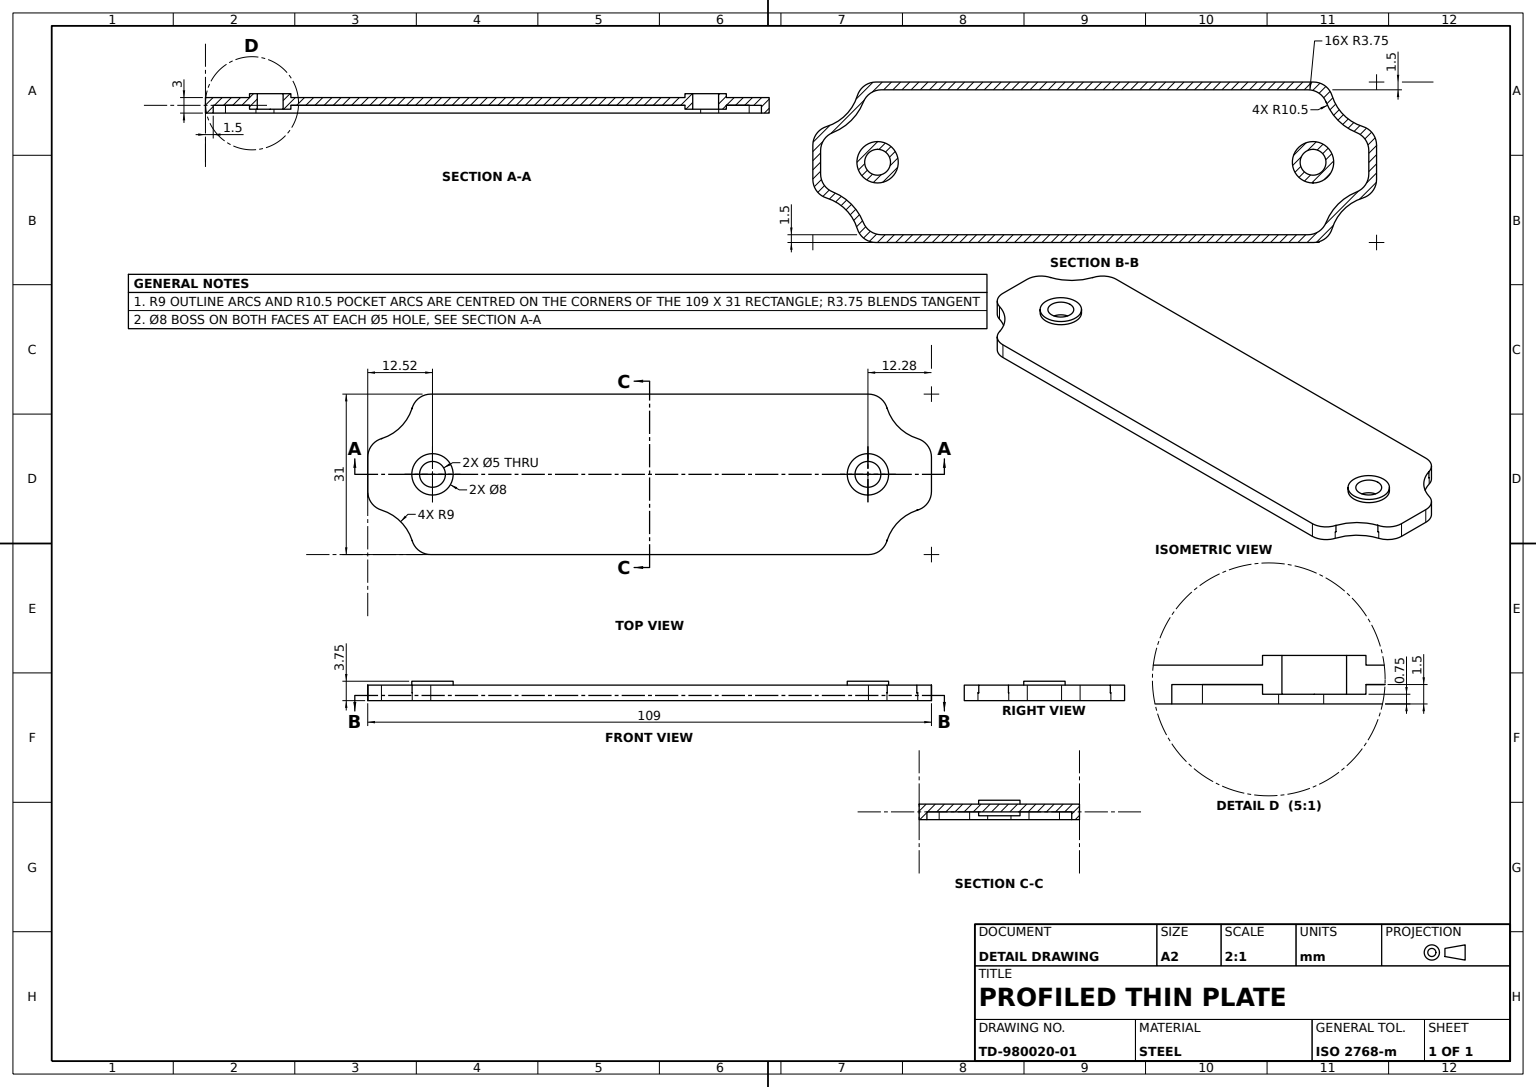
SolidWorks part; units mm, degrees
material "Plain Carbon Steel"
ref_plane "Front Plane" through (0, 0, 0) normal (0, 0, 1) x (1, 0, 0)
ref_plane "Top Plane" through (0, 0, 0) normal (0, 1, 0) x (1, 0, 0)
ref_plane "Right Plane" through (0, 0, 0) normal (1, 0, 0) x (0, 0, -1)
sketch "Plate Outline Sketch" plane through (0, 0, 0) normal (0, 1, 0) x (1, 0, 0)
  line L1 (-45.5, -15.5) -> (45.5, -15.5)
  line L2 (-54.5, -6.5) -> (-54.5, 6.5)
  line L3 (-45.5, 15.5) -> (45.5, 15.5)
  line L4 (54.5, -6.5) -> (54.5, 6.5)
  arc A0 (-54.5, 6.5) -> (-45.5, 15.5) centre (-54.5, 15.5) ccw
  arc A1 (45.5, 15.5) -> (54.5, 6.5) centre (54.5, 15.5) ccw
  arc A2 (54.5, -6.5) -> (45.5, -15.5) centre (54.5, -15.5) ccw
  arc A3 (-45.5, -15.5) -> (-54.5, -6.5) centre (-54.5, -15.5) ccw
  circle A4 centre (-41.9824, 0) radius 2.5
  circle A5 centre (42.2171, 0) radius 2.5
  point P0 (0, 0)
  point P17 (0, 0)
  dimension "D3" = 18
  dimension "D4" = 18
  dimension "D5" = 18
  dimension "D6" = 18
  dimension "D7" = 5
  dimension "D8" = 5
  dimension "D1" = 109
  dimension "D2" = 31
  dimension "D9" = 54.5
  dimension "D10" = 15.5
  dimension "D11" = 41.9824
  dimension "D12" = 42.2171
extrude "Base Plate 1.5mm" add sketch "Plate Outline Sketch" against normal blind 1.5
sketch "Underside Boss Sketch" plane through (0, 0, 0) normal (0, 1, 0) x (1, 0, 0)
  line L20 (42.3139, 15.5) -> (-42.3139, 15.5)
  line L21 (-54.5, 3.3139) -> (-54.5, -3.3139)
  line L22 (-42.3139, -15.5) -> (42.3139, -15.5)
  line L23 (54.5, -3.3139) -> (54.5, 3.3139)
  line L24 (53, -5.1077) -> (53, 5.1077)
  line L25 (-44.1077, -14) -> (44.1077, -14)
  line L26 (-53, 5.1077) -> (-53, -5.1077)
  line L27 (44.1077, 14) -> (-44.1077, 14)
  line L28 (53, -2.2524) -> (53, 2.2524)
  line L29 (-41.2524, -14) -> (41.2524, -14)
  line L30 (-53, 2.2524) -> (-53, -2.2524)
  line L31 (41.2524, 14) -> (-41.2524, 14)
  line L32 (44.1077, 14) -> (-44.1077, 14) construction
  line L33 (45.5, 15.5) -> (-45.5, 15.5) construction
  line L34 (54.5, -6.5) -> (54.5, 6.5) construction
  line L35 (53, -5.1077) -> (53, 5.1077) construction
  line L36 (-45.5, -15.5) -> (45.5, -15.5) construction
  line L37 (-44.1077, -14) -> (44.1077, -14) construction
  line L38 (-54.5, 6.5) -> (-54.5, -6.5) construction
  line L39 (-53, 5.1077) -> (-53, -5.1077) construction
  arc A17 (-51.8529, 6.8981) -> (-45.8981, 12.8529) centre (-54.5, 15.5) ccw
  arc A18 (-45.8981, -12.8529) -> (-51.8529, -6.8981) centre (-54.5, -15.5) ccw
  arc A19 (51.8529, -6.8981) -> (45.8981, -12.8529) centre (54.5, -15.5) ccw
  arc A20 (45.8981, 12.8529) -> (51.8529, 6.8981) centre (54.5, 15.5) ccw
  arc A21 (44.1077, 14) -> (53, 5.1077) centre (54.5, 15.5) ccw
  arc A22 (53, -5.1077) -> (44.1077, -14) centre (54.5, -15.5) ccw
  arc A23 (-44.1077, -14) -> (-53, -5.1077) centre (-54.5, -15.5) ccw
  arc A24 (-53, 5.1077) -> (-44.1077, 14) centre (-54.5, 15.5) ccw
  arc A25 (44.7386, 11.6316) -> (50.6316, 5.7386) centre (54.5, 15.5) ccw
  arc A26 (50.6316, -5.7386) -> (44.7386, -11.6316) centre (54.5, -15.5) ccw
  arc A27 (-44.7386, -11.6316) -> (-50.6316, -5.7386) centre (-54.5, -15.5) ccw
  arc A28 (-50.6316, 5.7386) -> (-44.7386, 11.6316) centre (-54.5, 15.5) ccw
  arc A29 (44.1077, 14) -> (53, 5.1077) centre (54.5, 15.5) ccw construction
  arc A30 (44.7386, 11.6316) -> (41.2524, 14) centre (41.2524, 10.25) ccw
  arc A31 (45.5, 15.5) -> (54.5, 6.5) centre (54.5, 15.5) ccw construction
  arc A32 (45.8981, 12.8529) -> (42.3139, 15.5) centre (42.3139, 11.75) ccw
  arc A33 (54.5, 3.3139) -> (51.8529, 6.8981) centre (50.75, 3.3139) ccw
  arc A34 (53, 2.2524) -> (50.6316, 5.7386) centre (49.25, 2.2524) ccw
  arc A35 (53, -5.1077) -> (44.1077, -14) centre (54.5, -15.5) ccw construction
  arc A36 (50.6316, -5.7386) -> (53, -2.2524) centre (49.25, -2.2524) ccw
  arc A37 (54.5, -6.5) -> (45.5, -15.5) centre (54.5, -15.5) ccw construction
  arc A38 (54.5, -3.3139) -> (51.8529, -6.8981) centre (50.75, -3.3139) cw
  arc A39 (42.3139, -15.5) -> (45.8981, -12.8529) centre (42.3139, -11.75) ccw
  arc A40 (41.2524, -14) -> (44.7386, -11.6316) centre (41.2524, -10.25) ccw
  arc A41 (-45.5, -15.5) -> (-54.5, -6.5) centre (-54.5, -15.5) ccw construction
  arc A42 (-42.3139, -15.5) -> (-45.8981, -12.8529) centre (-42.3139, -11.75) cw
  arc A43 (-44.1077, -14) -> (-53, -5.1077) centre (-54.5, -15.5) ccw construction
  arc A44 (-41.2524, -14) -> (-44.7386, -11.6316) centre (-41.2524, -10.25) cw
  arc A45 (-51.8529, -6.8981) -> (-54.5, -3.3139) centre (-50.75, -3.3139) cw
  arc A46 (-50.6316, -5.7386) -> (-53, -2.2524) centre (-49.25, -2.2524) cw
  arc A47 (-53, 5.1077) -> (-44.1077, 14) centre (-54.5, 15.5) ccw construction
  arc A48 (-53, 2.2524) -> (-50.6316, 5.7386) centre (-49.25, 2.2524) cw
  arc A49 (-54.5, 6.5) -> (-45.5, 15.5) centre (-54.5, 15.5) ccw construction
  arc A50 (-54.5, 3.3139) -> (-51.8529, 6.8981) centre (-50.75, 3.3139) cw
  arc A51 (-44.7386, 11.6316) -> (-41.2524, 14) centre (-41.2524, 10.25) cw
  arc A52 (-45.8981, 12.8529) -> (-42.3139, 15.5) centre (-42.3139, 11.75) cw
  dimension "D3" = 3.75
  dimension "D1" = 1.5
  dimension "D2" = 1.5
extrude "Underside Bosses" add sketch "Underside Boss Sketch" against normal blind 3
sketch "End Boss A Sketch" plane through (0, 0, 0) normal (0, 1, 0) x (1, 0, 0)
  circle A0 centre (-41.9824, 0) radius 4
  circle A1 centre (42.2171, 0) radius 4
  circle A2 centre (-41.9824, 0) radius 2.5
  circle A3 centre (42.2171, 0) radius 2.5
  dimension "D1" = 8
  dimension "D2" = 8
  dimension "D3" = 5
sketch "Through Hole Sketch" plane through (0, -1.5, 0) normal (0, -1, 0) x (1, 0, 0)
  line L0 (-42.3139, 15.5) -> (-45.5, 15.5)
  line L1 (-45.5, 15.5) -> (-45.9252, 12.7607)
  line L2 (42.3139, 15.5) -> (45.5, 15.5)
  line L3 (45.5, 15.5) -> (45.9566, 12.6407)
  line L4 (54.5, 3.3139) -> (54.5, 6.5)
  line L5 (54.5, 6.5) -> (51.5878, 6.9691)
  line L6 (51.8529, -6.8981) -> (54.5, -6.5)
  line L7 (54.5, -6.5) -> (54.5, -3.3139)
  line L8 (42.3139, -15.5) -> (45.5, -15.5)
  line L9 (45.5, -15.5) -> (45.9365, -12.7192)
  line L10 (-42.3139, -15.5) -> (-45.5, -15.5)
  line L11 (-45.5, -15.5) -> (-45.95, -12.6673)
  line L12 (-54.5, -3.3139) -> (-54.5, -6.5)
  line L13 (-54.5, -6.5) -> (-51.7139, -6.938)
  line L14 (-54.5, 3.3139) -> (-54.5, 6.5)
  line L15 (-54.5, 6.5) -> (-51.8529, 6.8981)
  arc A0 (-54.5, -3.3139) -> (-51.7139, -6.938) centre (-50.75, -3.3139) ccw
  arc A1 (45.9566, 12.6407) -> (42.3139, 15.5) centre (42.3139, 11.75) ccw
  arc A2 (54.5, 3.3139) -> (51.5878, 6.9691) centre (50.75, 3.3139) ccw
  arc A3 (51.8529, -6.8981) -> (54.5, -3.3139) centre (50.75, -3.3139) ccw
  arc A4 (42.3139, -15.5) -> (45.9365, -12.7192) centre (42.3139, -11.75) ccw
  arc A5 (-45.95, -12.6673) -> (-42.3139, -15.5) centre (-42.3139, -11.75) ccw
  arc A6 (-51.8529, 6.8981) -> (-54.5, 3.3139) centre (-50.75, 3.3139) ccw
  arc A7 (-42.3139, 15.5) -> (-45.9252, 12.7607) centre (-42.3139, 11.75) ccw
  dimension "D1" = 0.0385
  dimension "D2" = 0.0586
  dimension "D3" = 5.6898
  dimension "D4" = 91.8232
  dimension "D5" = 91.8481
  dimension "D6" = 97.6119
extrude "Through Holes" cut sketch "Through Hole Sketch" against normal blind 3
sketch "End Boss B Sketch" plane through (0, 0, 0) normal (0, 1, 0) x (1, 0, 0)
  circle A0 centre (-41.9824, 0) radius 4
  circle A1 centre (42.2171, 0) radius 4
  circle A2 centre (-41.9824, 0) radius 2.5
  circle A3 centre (42.2171, 0) radius 2.5
  dimension "D1" = 8
  dimension "D2" = 8
  dimension "D3" = 5
extrude "Raised End Boss B 8mm" add sketch "End Boss B Sketch" along normal blind 0.75 and the other way blind 2.25
extrude "Raised End Boss A 8mm" add sketch "End Boss A Sketch" along normal blind 0.75 and the other way blind 2.25
